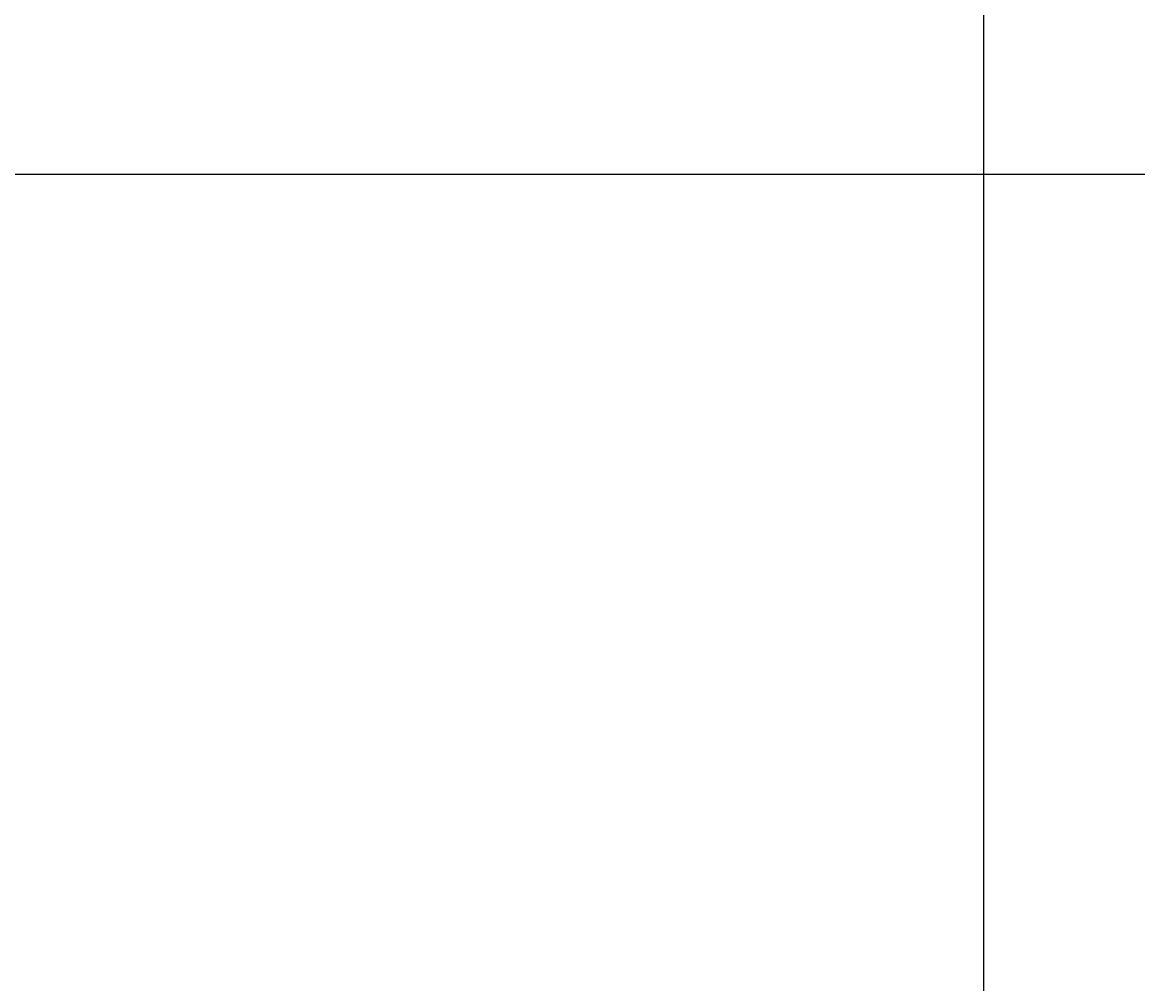
# Model space of a CAD drawing. Units: inches. Extents: x 35362 to 73946, y 43607 to 67532.
# Tile 109 of 134: x 50905 to 51049, y 48793 to 48917. Entities that reach past the tile are written whole.
import ezdxf

# ---------------------------------------------------------------- set-up
doc = ezdxf.new("R2010")
doc.units = ezdxf.units.IN
doc.header["$MEASUREMENT"] = 0
doc.layers.add('A-ANNO-DIMS', color=2, linetype='Continuous', lineweight=18)
doc.styles.get("Standard").update_dxf_attribs({"font": 'arial.ttf'})
doc.dimstyles.get("Standard").update_dxf_attribs({"dimtxt": 0.18, "dimasz": 0.18, "dimexe": 0.18, "dimexo": 0.0625, "dimgap": 0.09, "dimtad": 0, "dimtih": 1, "dimtoh": 1, "dimdec": 4, "dimzin": 0, "dimdsep": 46, "dimtxsty": 'Standard', "dimcen": 0.09, "dimadec": 0, "dimazin": 0, "dimtfac": 1, "dimtdec": 4, "dimtofl": 0, "dimtmove": 0, "dimatfit": 3, "dimfxl": 1, "dimtolj": 1, "dimtzin": 0, "dimarcsym": 0})

# ---------------------------------------------------------------- blocks, each defined once
blk = doc.blocks.new('*D11')
at = {"layer": 'A-ANNO-DIMS', "color": 0, "lineweight": -2, "transparency": 16777216}
for p, q in [((47978.66, 56028.77), (47978.66, 43606.68)), ((53109.76, 56028.77), (53109.76, 43606.68)), ((47978.84, 43606.86), (50543.87, 43606.86)), ((53109.58, 43606.86), (50544.55, 43606.86))]:
    blk.add_line(p, q, dxfattribs=at)
at = {"layer": 'A-ANNO-DIMS', "color": 0, "transparency": 16777216}
for points in [[(47978.84, 43606.89), (47978.84, 43606.83), (47978.66, 43606.86)], [(53109.58, 43606.89), (53109.58, 43606.83), (53109.76, 43606.86)]]:
    blk.add_solid(points, dxfattribs=at)
at = {"layer": 'Defpoints', "color": 0, "transparency": 16777216}
for p in [(47978.66, 56028.84), (53109.76, 56028.84), (53109.76, 43606.86)]:
    blk.add_point(p, dxfattribs=at)
at = {"layer": 'A-ANNO-DIMS', "color": 0, "transparency": 16777216, "insert": (50544.21, 43606.86), "char_height": 0.18, "attachment_point": 5}
blk.add_mtext('\\A1;5131', dxfattribs=at)
blk = doc.blocks.new('*D13')
at = {"layer": 'A-ANNO-DIMS', "color": 0, "lineweight": -2, "transparency": 16777216}
for p, q in [((48373.49, 51694.02), (48373.49, 43606.68)), ((51029.04, 51694.02), (51029.04, 43606.68)), ((48373.67, 43606.86), (49700.8, 43606.86)), ((51028.86, 43606.86), (49701.73, 43606.86))]:
    blk.add_line(p, q, dxfattribs=at)
at = {"layer": 'A-ANNO-DIMS', "color": 0, "transparency": 16777216}
for points in [[(48373.67, 43606.89), (48373.67, 43606.83), (48373.49, 43606.86)], [(51028.86, 43606.89), (51028.86, 43606.83), (51029.04, 43606.86)]]:
    blk.add_solid(points, dxfattribs=at)
at = {"layer": 'Defpoints', "color": 0, "transparency": 16777216}
for p in [(48373.49, 51694.09), (51029.04, 51694.09), (51029.04, 43606.86)]:
    blk.add_point(p, dxfattribs=at)
at = {"layer": 'A-ANNO-DIMS', "color": 0, "transparency": 16777216, "insert": (49701.27, 43606.86), "char_height": 0.18, "attachment_point": 5}
blk.add_mtext('\\A1;2655.6', dxfattribs=at)
blk = doc.blocks.new('*D17')
at = {"layer": 'A-ANNO-DIMS', "color": 0, "lineweight": -2, "transparency": 16777216}
for p, q in [((49923.31, 61293.22), (49923.31, 43606.68)), ((51913.93, 61293.22), (51913.93, 43606.68)), ((49923.49, 43606.86), (50918.16, 43606.86)), ((51913.75, 43606.86), (50919.07, 43606.86))]:
    blk.add_line(p, q, dxfattribs=at)
at = {"layer": 'A-ANNO-DIMS', "color": 0, "transparency": 16777216}
for points in [[(49923.49, 43606.89), (49923.49, 43606.83), (49923.31, 43606.86)], [(51913.75, 43606.89), (51913.75, 43606.83), (51913.93, 43606.86)]]:
    blk.add_solid(points, dxfattribs=at)
at = {"layer": 'Defpoints', "color": 0, "transparency": 16777216}
for p in [(49923.31, 61293.29), (51913.93, 61293.29), (51913.93, 43606.86)]:
    blk.add_point(p, dxfattribs=at)
at = {"layer": 'A-ANNO-DIMS', "color": 0, "transparency": 16777216, "insert": (50918.62, 43606.86), "char_height": 0.18, "attachment_point": 5}
blk.add_mtext('\\A1;1990.6', dxfattribs=at)
blk = doc.blocks.new('*D67')
at = {"layer": 'A-ANNO-DIMS', "color": 0, "lineweight": -2, "transparency": 16777216}
for p, q in [((56873.54, 53351.53), (35361.77, 53351.53)), ((35361.95, 53351.35), (35361.95, 49400.89)), ((35361.95, 45450.07), (35361.95, 49400.53)), ((53793.58, 45449.89), (35361.77, 45449.89))]:
    blk.add_line(p, q, dxfattribs=at)
at = {"layer": 'A-ANNO-DIMS', "color": 0, "transparency": 16777216}
for points in [[(35361.92, 53351.35), (35361.98, 53351.35), (35361.95, 53351.53)], [(35361.92, 45450.07), (35361.98, 45450.07), (35361.95, 45449.89)]]:
    blk.add_solid(points, dxfattribs=at)
at = {"layer": 'Defpoints', "color": 0, "transparency": 16777216}
for p in [(35361.95, 53351.53), (56873.6, 53351.53), (53793.64, 45449.89)]:
    blk.add_point(p, dxfattribs=at)
at = {"layer": 'A-ANNO-DIMS', "color": 0, "transparency": 16777216, "insert": (35361.95, 49400.71), "char_height": 0.18, "attachment_point": 5}
blk.add_mtext('\\A1;7901.6', dxfattribs=at)
blk = doc.blocks.new('*D89')
at = {"layer": 'A-ANNO-DIMS', "color": 0, "lineweight": -2, "transparency": 16777216}
for p, q in [((53707.72, 48897.74), (35361.77, 48897.74)), ((35361.95, 48897.56), (35361.95, 48303.16)), ((35361.95, 47708.4), (35361.95, 48302.8)), ((53707.72, 47708.22), (35361.77, 47708.22))]:
    blk.add_line(p, q, dxfattribs=at)
at = {"layer": 'A-ANNO-DIMS', "color": 0, "transparency": 16777216}
for points in [[(35361.92, 48897.56), (35361.98, 48897.56), (35361.95, 48897.74)], [(35361.92, 47708.4), (35361.98, 47708.4), (35361.95, 47708.22)]]:
    blk.add_solid(points, dxfattribs=at)
at = {"layer": 'Defpoints', "color": 0, "transparency": 16777216}
for p in [(53707.78, 48897.74), (35361.95, 47708.22), (53707.78, 47708.22)]:
    blk.add_point(p, dxfattribs=at)
at = {"layer": 'A-ANNO-DIMS', "color": 0, "transparency": 16777216, "insert": (35361.95, 48302.98), "char_height": 0.18, "attachment_point": 5}
blk.add_mtext('\\A1;1189.5', dxfattribs=at)
blk = doc.blocks.new('*D107')
at = {"layer": 'A-ANNO-DIMS', "color": 0, "lineweight": -2, "transparency": 16777216}
for p, q in [((50139.56, 59850.01), (50139.56, 43606.68)), ((51320.81, 59850.01), (51320.81, 43606.68)), ((50139.74, 43606.86), (50729.73, 43606.86)), ((51320.63, 43606.86), (50730.64, 43606.86))]:
    blk.add_line(p, q, dxfattribs=at)
at = {"layer": 'A-ANNO-DIMS', "color": 0, "transparency": 16777216}
for points in [[(50139.74, 43606.89), (50139.74, 43606.83), (50139.56, 43606.86)], [(51320.63, 43606.89), (51320.63, 43606.83), (51320.81, 43606.86)]]:
    blk.add_solid(points, dxfattribs=at)
at = {"layer": 'Defpoints', "color": 0, "transparency": 16777216}
for p in [(50139.56, 59850.08), (51320.81, 59850.08), (51320.81, 43606.86)]:
    blk.add_point(p, dxfattribs=at)
at = {"layer": 'A-ANNO-DIMS', "color": 0, "transparency": 16777216, "insert": (50730.19, 43606.86), "char_height": 0.18, "attachment_point": 5}
blk.add_mtext('\\A1;1181.3', dxfattribs=at)

msp = doc.modelspace()

# ---------------------------------------------------------------- dimensions: what is measured, and where the dimension line sits
at = {"layer": 'A-ANNO-DIMS'}
for base, p1, p2, override, picture, middle in [((51913.931, 43606.859), (49923.307, 61293.286), (51913.931, 61293.286), {"dimdec": 1, "dimlfac": 1, "dimrnd": 0, "dimzin": 0, "dimdsep": 46, "dimlunit": 2}, '*D17', (50918.619, 43606.859)), ((51320.8133, 43606.859), (50139.5627, 59850.0769), (51320.8133, 59850.0769), {"dimdec": 1, "dimlfac": 1, "dimrnd": 0, "dimzin": 0, "dimdsep": 46, "dimlunit": 2}, '*D107', (50730.188, 43606.859)), ((53109.76, 43606.859), (47978.665, 56028.836), (53109.76, 56028.836), {"dimdec": 0, "dimlfac": 1, "dimrnd": 0, "dimzin": 0, "dimdsep": 46, "dimlunit": 2}, '*D11', (50544.212, 43606.859)), ((51029.043, 43606.859), (48373.492, 51694.087), (51029.043, 51694.087), {"dimdec": 1, "dimlfac": 1, "dimrnd": 0, "dimzin": 0, "dimdsep": 46, "dimlunit": 2}, '*D13', (49701.267, 43606.859))]:
    dim = msp.add_linear_dim(base=base, p1=p1, p2=p2, dimstyle='Standard', override=override, dxfattribs=at)
    dim.commit()
    dim.dimension.update_dxf_attribs({"geometry": picture, "text_midpoint": middle})
for base, p1, p2, picture, middle in [((35361.949, 53351.529), (53793.638, 45449.894), (56873.602, 53351.529), '*D67', (35361.949, 49400.712)), ((35361.949, 47708.216), (53707.781, 48897.738), (53707.781, 47708.216), '*D89', (35361.949, 48302.977))]:
    dim = msp.add_linear_dim(base=base, p1=p1, p2=p2, angle=90, dimstyle='Standard', override={"dimdec": 1, "dimlfac": 1, "dimrnd": 0, "dimzin": 0, "dimdsep": 46, "dimlunit": 2}, dxfattribs=at)
    dim.commit()
    dim.dimension.update_dxf_attribs({"geometry": picture, "text_midpoint": middle})

doc.saveas('drawing.dxf')
